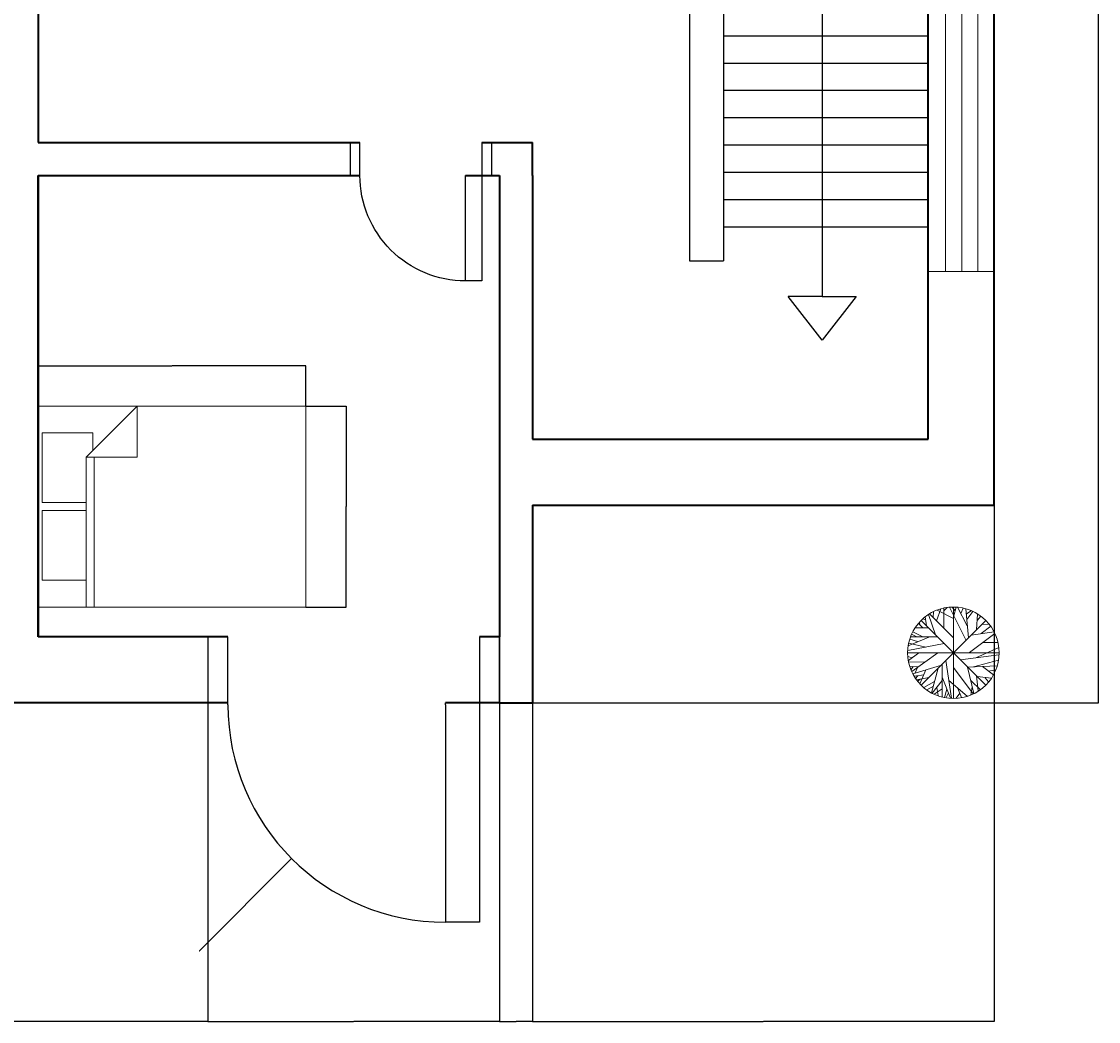
# Model space of a CAD drawing. Units: millimetres. Extents: x 726 to 37095, y -1634 to 13537.
# Tile 4 of 4: x 28928 to 37095, y -1634 to 5952. Entities that reach past the tile are written whole.
import ezdxf

# ---------------------------------------------------------------- set-up
doc = ezdxf.new("R2010")
doc.units = ezdxf.units.MM
for name, color, linetype, lineweight in [('A-ANNO-DIMS', 2, 'Continuous', 18), ('A-DOOR', 3, 'Continuous', 25), ('A-FLOR-STRS', 5, 'Continuous', 25), ('A-FURN', 8, 'Continuous', 18), ('A-GLAZ', 4, 'Continuous', 18), ('A-WALL', 7, 'Continuous', 35), ('L-PLNT', 94, 'Continuous', 18)]:
    doc.layers.add(name, color=color, linetype=linetype, lineweight=lineweight)
doc.styles.get("Standard").update_dxf_attribs({"font": 'arial.ttf'})
doc.dimstyles.get("Standard").update_dxf_attribs({"dimtxt": 0.18, "dimasz": 0.18, "dimexe": 0.18, "dimexo": 0.0625, "dimgap": 0.09, "dimtad": 0, "dimtih": 1, "dimtoh": 1, "dimdec": 4, "dimzin": 0, "dimdsep": 46, "dimtxsty": 'Standard', "dimcen": 0.09, "dimadec": 0, "dimazin": 0, "dimtfac": 1, "dimtdec": 4, "dimtofl": 0, "dimtmove": 0, "dimatfit": 3, "dimfxl": 1, "dimtolj": 1, "dimtzin": 0, "dimarcsym": 0})

# ---------------------------------------------------------------- blocks, each defined once
blk = doc.blocks.new('Window - Wood Frame 36 in. Wide plan')
for p, q in [((0, 6), (0, 0)), ((36, 6), (36, 0)), ((0, 4.5), (36, 4.5)), ((0, 3), (36, 3)), ((0, 1.5), (36, 1.5))]:
    blk.add_line(p, q)
blk = doc.blocks.new('Bed - Queen')
for p, q in [((0, -80.00003000000002), (0, 0)), ((0, 0), (59.99998999999999, 0)), ((59.99998999999999, 0), (59.99998999999999, -80.00003000000002)), ((7.99999, -1.200000000000017), (28.79998, -1.200000000000017)), ((7.99999, -14.4), (7.99999, -1.200000000000017)), ((28.79998, -1.200000000000017), (28.79998, -14.4)), ((31.19999, -1.200000000000017), (51.99999000000001, -1.200000000000017)), ((31.19999, -14.4), (31.19999, -1.200000000000017)), ((51.99999000000001, -1.200000000000017), (51.99999000000001, -16.4)), ((0, -14.4), (44.79999999999999, -14.4)), ((59.99998999999999, -29.60000000000001), (44.79999999999999, -14.4)), ((44.79999999999999, -14.4), (44.79999999999999, -29.60000000000001)), ((44.79999999999999, -16.80000000000001), (0, -16.80000000000001)), ((51.99999000000001, -16.4), (46.79936, -16.4)), ((44.79999999999999, -29.60000000000001), (59.99998999999999, -29.60000000000001)), ((59.99998999999999, -80.00003000000002), (0, -80.00003000000002))]:
    blk.add_line(p, q)
blk = doc.blocks.new('Tree - deciduous plan')
for p, q in [((-22.04579999999999, 42.07529999999986), (-16.58809999999994, 57.64859999999988)), ((-12.53879999999992, 54.94059999999979), (-7.961299999999937, 59.45459999999991)), ((-12.36270000000002, 32.14429999999993), (-12.53879999999992, 58.77760000000001)), ((-5.320499999999924, 59.68059999999979), (16.51049999999998, 16.79629999999986)), ((2.426000000000044, 54.94059999999979), (-1.447199999999952, 59.90559999999982)), ((0, 59.99959999999987), (0, -60.00000000000011)), ((0.4894000000000461, 48.62079999999991), (3.658400000000028, 59.68059999999979)), ((18.27110000000004, 35.52979999999991), (5.418999999999982, 59.68059999999979)), ((9.820299999999975, 51.55489999999986), (12.81330000000002, 58.55159999999989)), ((19.67950000000007, 19.50469999999984), (16.33440000000007, 57.64859999999988)), ((-40.17970000000002, 44.55799999999988), (-36.48249999999996, 43.20379999999988)), ((-37.01069999999993, 47.04079999999987), (-35.25, 35.52979999999991)), ((-32.60919999999999, 50.42639999999995), (-23.27819999999997, 23.56739999999991)), ((-31.20079999999996, 51.10349999999994), (-0.2148999999999432, 20.18179999999984)), ((-26.44719999999995, 46.58939999999984), (-26.27120000000002, 53.81159999999988)), ((-21.16559999999993, 55.84359999999981), (-0.0387999999999238, 45.00939999999991)), ((17.03870000000006, 51.10349999999994), (23.20060000000001, 55.16659999999991)), ((17.74290000000007, 43.65519999999992), (25.48940000000005, 54.26359999999988)), ((31.65129999999999, 50.87779999999987), (30.24290000000008, 30.56429999999989)), ((31.1232, 42.52669999999989), (35.87670000000003, 48.16929999999991)), ((-49.86270000000001, 32.82139999999993), (-32.78530000000001, 32.82139999999993)), ((-45.81339999999999, 38.23829999999987), (-40.53179999999997, 33.04709999999989)), ((-43.8768, 36.43259999999998), (-44.40499999999997, 40.26959999999997)), ((42, 41.99999999999988), (-42, -42.00000000000011)), ((42, -42.00000000000011), (-42, 41.99999999999988)), ((36.22879999999998, 25.14739999999995), (48.90489999999999, 35.07839999999987)), ((37.10910000000001, 37.10979999999995), (46.61609999999996, 37.56119999999987)), ((-32.25709999999992, 20.63329999999985), (-59.19370000000004, 9.347999999999843)), ((-57.08100000000001, 17.92479999999989), (-47.04579999999999, 14.7648999999999)), ((-56.02469999999994, 20.85899999999992), (-20.8134, 20.85899999999992)), ((-54.79229999999995, 24.47019999999986), (-47.75, 21.08469999999988)), ((-53.20780000000002, 27.4043999999999), (-40.17970000000002, 20.85899999999992)), ((54.36260000000004, 25.37309999999991), (20.91190000000006, 0.3197999999998728)), ((23.37670000000003, 23.34169999999994), (53.30629999999996, 27.4043999999999)), ((-59.72190000000001, 2.802499999999895), (-12.01059999999995, 12.05649999999991)), ((-58.66559999999992, 12.73359999999991), (-35.95429999999999, 7.542399999999929)), ((-54.61619999999993, -24.73350000000016), (-20.28530000000001, 0.0940999999999122)), ((29.36260000000004, -6.677100000000109), (59.46820000000002, 7.090999999999894)), ((38.51750000000004, 13.4106999999999), (58.23590000000002, 13.63639999999987)), ((-60, -1.137e-13), (60, -1.137e-13)), ((-59.72190000000001, -4.871400000000107), (-54.26409999999998, -6.677100000000109)), ((-45.2853, -0.1316000000001622), (-59.01769999999999, -10.06270000000006)), ((-58.48950000000002, -12.31970000000012), (-36.48249999999996, -11.64260000000013)), ((-10.07399999999995, -10.06270000000006), (-2.503600000000005, -59.71780000000013)), ((9.29219999999998, -9.159800000000132), (59.64430000000004, -2.84010000000012)), ((26.36969999999997, -18.41380000000015), (58.94010000000003, -9.836900000000128)), ((-57.08100000000001, -18.41380000000015), (-45.2853, -17.9624)), ((-52.67970000000002, -18.1880000000001), (-55.49659999999994, -22.02510000000007)), ((-53.20780000000002, -27.44200000000012), (-16.76409999999998, -16.60810000000015)), ((-47.2219, -19.31660000000011), (-50.21479999999996, -26.31350000000009)), ((-35.95429999999999, -22.4765000000001), (-44.05290000000002, -40.53290000000015)), ((-19.93309999999997, -20.21940000000018), (-28.55989999999997, -52.72100000000012)), ((-14.82749999999998, -15.02820000000008), (-14.65149999999994, -57.68650000000014)), ((-0.0387999999999238, -19.09090000000015), (25.8415, -53.84950000000015)), ((18.6232, -18.63940000000013), (26.72180000000003, -53.39810000000011)), ((18.79920000000004, -18.63940000000013), (57.35559999999998, -17.28530000000012)), ((38.16539999999998, -18.1880000000001), (52.42600000000004, -29.02190000000008)), ((45.91190000000006, -24.05640000000017), (55.59500000000003, -22.25080000000014)), ((-38.94719999999995, -29.02190000000008), (-51.44719999999995, -30.60180000000014)), ((-46.51769999999999, -30.15040000000011), (-49.51059999999995, -33.53600000000006)), ((-32.43309999999997, -32.40750000000014), (-48.10209999999995, -35.56740000000002)), ((-43.70079999999996, -34.66450000000009), (-46.69370000000003, -37.37300000000016)), ((-24.68669999999998, -37.8244000000002), (-38.77120000000002, -45.72410000000013)), ((-14.65149999999994, -36.24450000000013), (-27.67970000000003, -52.94670000000007)), ((-14.65149999999994, -32.18180000000007), (-3.912000000000034, -59.49220000000014)), ((-6.200799999999958, -36.24450000000013), (17.91899999999998, -57.00940000000014)), ((22.84850000000006, -36.47020000000009), (35.34850000000006, -48.43260000000009)), ((30.41899999999998, -30.15040000000011), (32.35559999999998, -50.01250000000016)), ((31.47530000000006, -31.27900000000011), (49.60910000000001, -33.3103000000001)), ((41.51049999999997, -32.6332000000001), (46.08799999999996, -38.05010000000016)), ((-26.27120000000002, -43.91850000000011), (-34.72190000000001, -48.65830000000006)), ((-14.65149999999994, -47.30410000000006), (-25.03879999999993, -54.30090000000006)), ((-21.51769999999999, -45.49840000000005), (-19.93309999999997, -56.1065000000001)), ((-8.48950000000002, -47.52980000000014), (-11.48249999999996, -58.58930000000009)), ((-6.376800000000002, -52.72100000000012), (-9.369799999999941, -58.81500000000006)), ((8.41190000000006, -53.17240000000004), (3.834400000000073, -59.49220000000014)), ((5.947099999999977, -46.62690000000009), (10.52459999999996, -58.58930000000009)), ((24.78520000000003, -44.82130000000006), (23.02459999999996, -54.97800000000006))]:
    blk.add_line(p, q)
blk.add_circle((0, -1.137e-13), 60)
blk = doc.blocks.new('STAIR-QUARTER-TURN')
for p, q in [((1551.94660387568, 5000.000000000002), (1551.94660387568, 3551.516503049365)), ((1758.872817725773, 5000.000000000002), (1758.872817725773, 3551.516503049365)), ((1965.799031575862, 5000.000000000002), (1965.799031575862, 3551.516503049365)), ((2172.725245425954, 5000.000000000002), (2172.725245425954, 3551.516503049365)), ((2172.725245425954, 4193.579423830473), (803.743340616409, 4193.579423830471)), ((803.743340616409, 4193.579423830471), (803.743340616409, 330.5564002077117)), ((2172.725245425954, 3551.516503049366), (0, 3551.516503049365)), ((1551.94660387568, 3551.516503049365), (1551.94660387568, 3344.590289199272)), ((2172.725245425954, 3551.516503049365), (2172.725245425954, 3292.858735736751)), ((1551.94660387568, 3344.590289199272), (0, 3344.590289199273)), ((1551.94660387568, 3344.590289199272), (1551.94660387568, 861.4757229981805)), ((2172.725245425954, 3292.858735736751), (1810.604371188295, 3292.858735736751)), ((1810.604371188295, 3292.85873573675), (1810.604371188295, 602.8179556856148)), ((1551.94660387568, 3137.664075349182), (0, 3137.664075349182)), ((1551.94660387568, 2930.73786149909), (0, 2930.737861499091)), ((1551.94660387568, 2723.811647649), (0, 2723.811647649001)), ((1551.94660387568, 2516.885433798908), (0, 2516.885433798909)), ((1551.94660387568, 2309.959219948817), (0, 2309.959219948818)), ((1551.94660387568, 2103.033006098726), (0, 2103.033006098727)), ((1551.94660387568, 1896.106792248635), (0, 1896.106792248635)), ((1551.94660387568, 1689.180578398543), (0, 1689.180578398544)), ((1551.94660387568, 1482.254364548453), (0, 1482.254364548454)), ((1551.94660387568, 1275.328150698362), (0, 1275.328150698363)), ((1551.94660387568, 1068.40193684827), (0, 1068.401936848271)), ((1551.94660387568, 861.4757229981795), (0, 861.4757229981805)), ((1551.94660387568, 861.4757229981805), (1551.946603875687, 602.8179556856074)), ((1810.604371188295, 602.8179556856148), (1551.946603875687, 602.8179556855675)), ((803.743340616409, 330.5564002077117), (545.0855733037969, 330.5564002077117)), ((545.0855733037969, 330.5564002077117), (803.743340616409, 4.547e-13)), ((803.743340616409, 330.5564002077117), (1062.401107929021, 330.5564002077108)), ((803.743340616409, 4.547e-13), (1062.401107929021, 330.5564002077117))]:
    blk.add_line(p, q)
blk = doc.blocks.new('*D23')
at = {"layer": 'A-ANNO-DIMS', "color": 0, "lineweight": -2, "transparency": 16777216}
for p, q in [((29053.4000535186, 3033.948368122885), (29053.4000535186, 3338.865982422885)), ((29053.5800535186, 3338.685982422885), (30067.95718076689, 3338.685982422885)), ((31085.2208155186, 3338.685982422885), (30070.84368827031, 3338.685982422885)), ((31085.4008155186, 3033.948368122885), (31085.4008155186, 3338.865982422885))]:
    blk.add_line(p, q, dxfattribs=at)
at = {"layer": 'A-ANNO-DIMS', "color": 0, "transparency": 16777216}
for points in [[(29053.5800535186, 3338.715982422885), (29053.5800535186, 3338.655982422885), (29053.4000535186, 3338.685982422885)], [(31085.2208155186, 3338.715982422885), (31085.2208155186, 3338.655982422885), (31085.4008155186, 3338.685982422885)]]:
    blk.add_solid(points, dxfattribs=at)
at = {"layer": 'Defpoints', "color": 0, "transparency": 16777216}
for p in [(29053.4000535186, 3338.685982422885), (29053.4000535186, 3033.885868122885), (31085.4008155186, 3033.885868122885)]:
    blk.add_point(p, dxfattribs=at)
at = {"layer": 'A-ANNO-DIMS', "color": 0, "transparency": 16777216, "insert": (30069.4004345186, 3338.685982422885), "char_height": 0.18, "attachment_point": 5}
blk.add_mtext('\\A1;QUEEN BED 2032 TYP.', dxfattribs=at)
blk = doc.blocks.new('*D24')
at = {"layer": 'A-ANNO-DIMS', "color": 0, "lineweight": -2, "transparency": 16777216}
for p, q in [((31085.46331551861, 3033.885868122885), (31390.38092981863, 3033.885868122885)), ((31390.20092981863, 3033.705868122885), (31390.20092981863, 2272.067898260676)), ((31390.20092981863, 1510.066122122885), (31390.20092981863, 2271.704091985096)), ((31085.46331551861, 1509.886122122885), (31390.38092981863, 1509.886122122886))]:
    blk.add_line(p, q, dxfattribs=at)
at = {"layer": 'A-ANNO-DIMS', "color": 0, "transparency": 16777216}
for points in [[(31390.17092981863, 3033.705868122885), (31390.23092981863, 3033.705868122885), (31390.20092981863, 3033.885868122885)], [(31390.17092981863, 1510.066122122885), (31390.23092981863, 1510.066122122885), (31390.20092981863, 1509.886122122886)]]:
    blk.add_solid(points, dxfattribs=at)
at = {"layer": 'Defpoints', "color": 0, "transparency": 16777216}
for p in [(31085.40081551861, 3033.885868122885), (31390.20092981863, 3033.885868122885), (31085.40081551861, 1509.886122122885)]:
    blk.add_point(p, dxfattribs=at)
at = {"layer": 'A-ANNO-DIMS', "color": 0, "transparency": 16777216, "insert": (31390.20092981862, 2271.885995122877), "char_height": 0.18, "attachment_point": 5}
blk.add_mtext('\\A1;1524 TYP.', dxfattribs=at)
blk = doc.blocks.new('*D64')
at = {"layer": 'A-ANNO-DIMS', "color": 0, "lineweight": -2, "transparency": 16777216}
for p, q in [((36303.46255400001, 12783.885868), (37094.80752400003, 12783.88586800001)), ((37094.62752400003, 12783.70586800001), (37094.62752400003, 6784.067771137793)), ((37094.62752400003, 784.065868000001), (37094.62752400003, 6783.703964862214)), ((32803.46255400001, 783.8858680000003), (37094.80752400003, 783.8858680000011))]:
    blk.add_line(p, q, dxfattribs=at)
at = {"layer": 'A-ANNO-DIMS', "color": 0, "transparency": 16777216}
for points in [[(37094.59752400003, 12783.70586800001), (37094.65752400003, 12783.70586800001), (37094.62752400003, 12783.88586800001)], [(37094.59752400003, 784.065868000001), (37094.65752400003, 784.065868000001), (37094.62752400003, 783.8858680000011)]]:
    blk.add_solid(points, dxfattribs=at)
at = {"layer": 'Defpoints', "color": 0, "transparency": 16777216}
for p in [(36303.40005400001, 12783.885868), (32803.40005400002, 783.8858680000003), (37094.62752400003, 783.8858680000011)]:
    blk.add_point(p, dxfattribs=at)
at = {"layer": 'A-ANNO-DIMS', "color": 0, "transparency": 16777216, "insert": (37094.62752400003, 6783.885867999991), "char_height": 0.18, "attachment_point": 5}
blk.add_mtext('\\A1;12000', dxfattribs=at)
blk = doc.blocks.new('*D66')
at = {"layer": 'A-ANNO-DIMS', "color": 0, "lineweight": -2, "transparency": 16777216}
for p, q in [((32803.400054, 2283.823368), (32803.400054, -1633.776092999999)), ((36303.400054, 2283.823368), (36303.400054, -1633.776092999999)), ((32803.580054, -1633.596093), (34553.04165018008, -1633.596093)), ((36303.220054, -1633.596093), (34553.75845781992, -1633.596093))]:
    blk.add_line(p, q, dxfattribs=at)
at = {"layer": 'A-ANNO-DIMS', "color": 0, "transparency": 16777216}
for points in [[(32803.580054, -1633.566093), (32803.580054, -1633.626093), (32803.400054, -1633.596093)], [(36303.220054, -1633.566093), (36303.220054, -1633.626093), (36303.400054, -1633.596093)]]:
    blk.add_solid(points, dxfattribs=at)
at = {"layer": 'Defpoints', "color": 0, "transparency": 16777216}
for p in [(32803.400054, 2283.885868), (36303.400054, 2283.885868), (36303.400054, -1633.596093)]:
    blk.add_point(p, dxfattribs=at)
at = {"layer": 'A-ANNO-DIMS', "color": 0, "transparency": 16777216, "insert": (34553.400054, -1633.596093), "char_height": 0.18, "attachment_point": 5}
blk.add_mtext('\\A1;3500', dxfattribs=at)
blk = doc.blocks.new('*D74')
at = {"layer": 'A-ANNO-DIMS', "color": 0, "lineweight": -2, "transparency": 16777216}
for p, q in [((32553.400054, 1283.823368), (32553.400054, -1633.776093)), ((32803.400054, 783.823368), (32803.400054, -1633.776092999999)), ((32553.580054, -1633.596093), (32678.10997896589, -1633.596093)), ((32803.220054, -1633.596093), (32678.6901290341, -1633.596093))]:
    blk.add_line(p, q, dxfattribs=at)
at = {"layer": 'A-ANNO-DIMS', "color": 0, "transparency": 16777216}
for points in [[(32553.580054, -1633.566093), (32553.580054, -1633.626093), (32553.400054, -1633.596093)], [(32803.220054, -1633.566093), (32803.220054, -1633.626093), (32803.400054, -1633.596093)]]:
    blk.add_solid(points, dxfattribs=at)
at = {"layer": 'Defpoints', "color": 0, "transparency": 16777216}
for p in [(32553.400054, 1283.885868), (32803.400054, 783.8858679999998), (32803.400054, -1633.596093)]:
    blk.add_point(p, dxfattribs=at)
at = {"layer": 'A-ANNO-DIMS', "color": 0, "transparency": 16777216, "insert": (32678.400054, -1633.596093), "char_height": 0.18, "attachment_point": 5}
blk.add_mtext('\\A1;250', dxfattribs=at)
blk = doc.blocks.new('*D83')
at = {"layer": 'A-ANNO-DIMS', "color": 0, "lineweight": -2, "transparency": 16777216}
for p, q in [((27354.503903, 783.523524), (27354.503903, -1633.776093)), ((30340.425495, 783.823368), (30340.425495, -1633.776092999999)), ((27354.683903, -1633.596093), (28847.10445343383, -1633.596093)), ((30340.245495, -1633.596093), (28847.82494456617, -1633.596093))]:
    blk.add_line(p, q, dxfattribs=at)
at = {"layer": 'A-ANNO-DIMS', "color": 0, "transparency": 16777216}
for points in [[(27354.683903, -1633.566093), (27354.683903, -1633.626093), (27354.503903, -1633.596093)], [(30340.245495, -1633.566093), (30340.245495, -1633.626093), (30340.425495, -1633.596093)]]:
    blk.add_solid(points, dxfattribs=at)
at = {"layer": 'Defpoints', "color": 0, "transparency": 16777216}
for p in [(27354.503903, 783.586024), (30340.425495, 783.8858679999998), (30340.425495, -1633.596093)]:
    blk.add_point(p, dxfattribs=at)
at = {"layer": 'A-ANNO-DIMS', "color": 0, "transparency": 16777216, "insert": (28847.464699, -1633.596093), "char_height": 0.18, "attachment_point": 5}
blk.add_mtext('\\A1;2986', dxfattribs=at)
blk = doc.blocks.new('*D84')
at = {"layer": 'A-ANNO-DIMS', "color": 0, "lineweight": -2, "transparency": 16777216}
for p, q in [((30340.425495, 1283.823368), (30340.425495, -1633.776093)), ((32553.400054, 1283.823368), (32553.400054, -1633.776093)), ((30340.605495, -1633.596093), (31446.55246754229, -1633.596093)), ((32553.220054, -1633.596093), (31447.27308145771, -1633.596093))]:
    blk.add_line(p, q, dxfattribs=at)
at = {"layer": 'A-ANNO-DIMS', "color": 0, "transparency": 16777216}
for points in [[(30340.605495, -1633.566093), (30340.605495, -1633.626093), (30340.425495, -1633.596093)], [(32553.220054, -1633.566093), (32553.220054, -1633.626093), (32553.400054, -1633.596093)]]:
    blk.add_solid(points, dxfattribs=at)
at = {"layer": 'Defpoints', "color": 0, "transparency": 16777216}
for p in [(30340.425495, 1283.885868), (32553.400054, 1283.885868), (32553.400054, -1633.596093)]:
    blk.add_point(p, dxfattribs=at)
at = {"layer": 'A-ANNO-DIMS', "color": 0, "transparency": 16777216, "insert": (31446.9127745, -1633.596093), "char_height": 0.18, "attachment_point": 5}
blk.add_mtext('\\A1;2213', dxfattribs=at)
blk = doc.blocks.new('*D89')
at = {"layer": 'A-ANNO-DIMS', "color": 0, "lineweight": -2, "transparency": 16777216}
for p, q in [((32142.629476, 768.4734970000026), (32142.809476, 768.4734970000007)), ((32142.719476, 768.3834969999988), (32142.719476, 768.5634969999973)), ((30276.72738686459, -1097.518625735425), (30976.34714078054, -397.8988592217575)), ((30276.54738686458, -1097.518625735425), (30276.72738686459, -1097.518625735425))]:
    blk.add_line(p, q, dxfattribs=at)
at = {"layer": 'A-ANNO-DIMS', "color": 0, "transparency": 16777216}
blk.add_solid([(30976.32592757692, -397.8776460185145), (30976.36835398417, -397.9200724250022), (30976.47442000001, -397.7715799999969)], dxfattribs=at)
at = {"layer": 'Defpoints', "color": 0, "transparency": 16777216}
for p in [(32142.719476, 768.4734970000007), (30976.47442000001, -397.7715799999969)]:
    blk.add_point(p, dxfattribs=at)
at = {"layer": 'A-ANNO-DIMS', "color": 0, "transparency": 16777216, "insert": (30275.99762560946, -1097.518625735427), "char_height": 0.18, "attachment_point": 5}
blk.add_mtext('\\A1;R1649.3', dxfattribs=at)

msp = doc.modelspace()

# ---------------------------------------------------------------- linework, layer by layer
at = {"layer": 'A-DOOR'}
for p, q in [((31494.61779927841, 5033.885868122884), (31420.41779927842, 5033.885868122882)), ((32493.81779927842, 5033.885868122886), (32419.61779927842, 5033.885868122886)), ((30493.39988677571, 1283.885868122885), (30340.42549488988, 1283.885868122885)), ((30340.42549488988, 1283.885868122885), (30340.42549488988, 783.8858681228854)), ((30493.39988677571, 768.4734965398984), (30493.39988677571, 1283.885868122885)), ((32553.40005351859, 1283.885868122885), (32400.42566163277, 1283.885868122885)), ((32400.42566163277, 1283.885868122885), (32400.42566163277, 768.4734965398984)), ((32553.40005351859, 783.8858681228851), (32553.40005351859, 1283.885868122885)), ((32142.71947584127, 768.4734965398984), (32142.71947584126, 783.8858681228851)), ((32142.71947584127, 768.4734965398984), (32142.71947584127, -880.8460925256575)), ((32400.42566163277, 768.4734965398984), (32400.42566163277, -880.8460925256575)), ((32400.42566163277, -880.8460925256575), (32142.71947584127, -880.8460925256575))]:
    msp.add_line(p, q, dxfattribs=at)
for points in [[(31346.21779927842, 5033.885868122887), (31420.41779927842, 5033.885868122889)], [(31494.61779927841, 4783.885868122886), (31494.61779927841, 5033.885868122886), (31420.41779927842, 5033.885868122886), (31420.41779927842, 4783.885868122886)], [(31494.61779927841, 5033.885868122887), (31420.41779927842, 5033.885868122889)]]:
    msp.add_lwpolyline(points, close=True, dxfattribs=at)
msp.add_lwpolyline([(31420.41779927842, 5033.885868122886), (31420.41779927842, 4783.885868122886)], dxfattribs=at)
msp.add_lwpolyline([(32294.61779927842, 3983.885868122886), (32294.61779927842, 4783.885868122886), (32419.61779927842, 4783.885868122886), (32493.81779927842, 4783.885868122886), (32493.81779927842, 5033.885868122886), (32419.61779927842, 5033.885868122886), (32419.61779927842, 4783.885868122886), (32419.61779927842, 3983.885868122886), (32294.61779927842, 3983.885868122886, -0.4142135623730951), (31494.61779927841, 4783.885868122886)], format="xyb", dxfattribs=at)
msp.add_arc((32142.71947584127, 768.4734965398984), 1649.319589065556, 180, 270, dxfattribs=at)
at = {"layer": 'A-WALL'}
for p, q in [((36303.40005351859, 2283.885868122886), (36303.40005351859, 12783.88586812288)), ((29053.4000535186, 8533.885868122885), (29053.4000535186, 5033.885868122885)), ((35803.40005351859, 2783.885868122886), (35803.40005351859, 8533.885868122885)), ((29053.4000535186, 5033.885868122886), (31494.61779927841, 5033.885868122886)), ((32419.61779927842, 5033.885868122886), (32553.4000535186, 5033.885868122886)), ((32553.4000535186, 5033.885868122886), (32803.40005351859, 5033.885868122886)), ((32803.40005351859, 4783.885868122886), (32803.40005351859, 5033.885868122886)), ((29053.4000535186, 1283.885868122886), (29053.4000535186, 4783.885868122886)), ((29053.4000535186, 4783.885868122886), (31494.61779927841, 4783.885868122886)), ((29053.4000535186, 4783.885868122886), (29053.4000535186, 1283.885868122886)), ((32294.61779927842, 4783.885868122886), (32553.4000535186, 4783.885868122886)), ((32553.4000535186, 4783.885868122886), (32553.4000535186, 1283.885868122885)), ((32803.40005351859, 4783.885868122886), (32803.40005351859, 2783.885868122885)), ((32803.40005351859, 2783.885868122886), (35803.40005351859, 2783.885868122886)), ((32803.40005351859, 2283.885868122885), (36303.40005351859, 2283.885868122886)), ((32803.40005351859, 2283.885868122885), (32803.40005351859, 1283.885868122885)), ((30493.39988677571, 1283.885868122885), (29053.4000535186, 1283.885868122886)), ((32553.4000535186, 1283.885868122885), (32400.42566163277, 1283.885868122885)), ((32803.40005351859, 1283.885868122885), (32803.40005351859, 1033.885868122885)), ((32803.40005351859, 1033.885868122885), (32803.40005351859, 783.8858681228851)), ((29053.4000535186, 783.8858681228855), (28553.40005351859, 783.8858681228857)), ((30493.39988677571, 783.8858681228854), (29053.4000535186, 783.8858681228855)), ((32553.4000535186, 783.8858681228851), (32142.71947584127, 783.8858681228852)), ((32553.4000535186, 783.8858681228851), (32803.40005351859, 783.8858681228847))]:
    msp.add_line(p, q, dxfattribs=at)

# ---------------------------------------------------------------- block references
at = {"layer": 'A-FLOR-STRS', "extrusion": (0, 0, -1), "zscale": -1}
msp.add_blockref('STAIR-QUARTER-TURN', (-35803.4000535186, 3533.885868122887), dxfattribs=at)
at = {"layer": 'A-FURN', "xscale": 25.4, "yscale": 25.4, "zscale": 25.4, "rotation": 90}
msp.add_blockref('Bed - Queen', (29053.4000535186, 1509.886122122885), dxfattribs=at)
at = {"layer": 'A-GLAZ', "xscale": 81.8978551733564, "yscale": 81.8978551733564, "zscale": 81.8978551733564, "rotation": 270}
msp.add_blockref('Window - Wood Frame 36 in. Wide plan', (35812.01292247845, 7003.139441062607), dxfattribs=at)
at = {"layer": 'L-PLNT', "xscale": 5.782335430308843, "yscale": 5.782335430308843, "zscale": 5.782335430308843}
msp.add_blockref('Tree - deciduous plan', (35994.9373981533, 1162.915302471572), dxfattribs=at)

# ---------------------------------------------------------------- dimensions: what is measured, and where the dimension line sits
at = {"layer": 'A-ANNO-DIMS'}
dim = msp.add_linear_dim(base=(37094.62752400003, 783.8858680000011), p1=(36303.400054, 12783.885868), p2=(32803.400054, 783.8858679999998), angle=90, dimstyle='Standard', override={"dimdec": 0, "dimlfac": 1, "dimrnd": 0, "dimzin": 0, "dimdsep": 46, "dimlunit": 2}, dxfattribs=at)
dim.commit()
dim.dimension.update_dxf_attribs({"geometry": '*D64', "text_midpoint": (37094.62752400003, 6783.885867999991)})
for base, p1, p2, angle, text, picture, middle in [((29053.4000535186, 3338.685982422885), (31085.4008155186, 3033.885868122885), (29053.4000535186, 3033.885868122885), 180, 'QUEEN BED <> TYP.', '*D23', (30069.4004345186, 3338.685982422885)), ((31390.20092981863, 3033.885868122885), (31085.4008155186, 1509.886122122885), (31085.4008155186, 3033.885868122885), 90, '<> TYP.', '*D24', (31390.20092981862, 2271.885995122877))]:
    dim = msp.add_linear_dim(base=base, p1=p1, p2=p2, angle=angle, text=text, dimstyle='Standard', override={"dimdec": 0, "dimlfac": 1, "dimrnd": 0, "dimzin": 0, "dimdsep": 46, "dimlunit": 2}, dxfattribs=at)
    dim.commit()
    dim.dimension.update_dxf_attribs({"geometry": picture, "text_midpoint": middle})
for base, p1, p2, picture, middle in [((36303.400054, -1633.596093), (32803.400054, 2283.885868), (36303.400054, 2283.885868), '*D66', (34553.400054, -1633.596093)), ((32553.400054, -1633.596093), (30340.425495, 1283.885868), (32553.400054, 1283.885868), '*D84', (31446.9127745, -1633.596093)), ((32803.400054, -1633.596093), (32553.400054, 1283.885868), (32803.400054, 783.8858679999998), '*D74', (32678.400054, -1633.596093)), ((30340.425495, -1633.596093), (27354.503903, 783.586024), (30340.425495, 783.8858679999998), '*D83', (28847.464699, -1633.596093))]:
    dim = msp.add_linear_dim(base=base, p1=p1, p2=p2, dimstyle='Standard', override={"dimdec": 0, "dimlfac": 1, "dimrnd": 0, "dimzin": 0, "dimdsep": 46, "dimlunit": 2}, dxfattribs=at)
    dim.commit()
    dim.dimension.update_dxf_attribs({"geometry": picture, "text_midpoint": middle})
dim = msp.add_radius_dim(center=(32142.719476, 768.4734970000007), mpoint=(30976.47442000001, -397.7715799999969), dimstyle='Standard', override={"dimdec": 1, "dimlfac": 1, "dimrnd": 0, "dimzin": 0, "dimdsep": 46, "dimlunit": 2}, dxfattribs=at)
dim.commit()
dim.dimension.update_dxf_attribs({"geometry": '*D89', "text_midpoint": (30275.99762560946, -1097.518625735427), "dimtype": 164})

doc.saveas('drawing.dxf')
